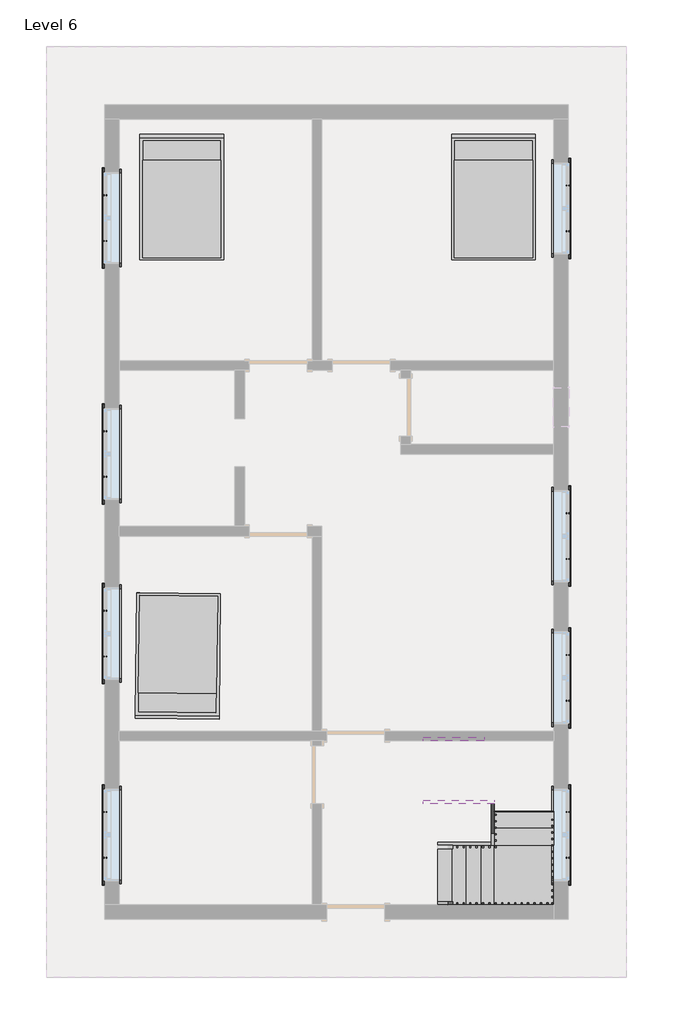
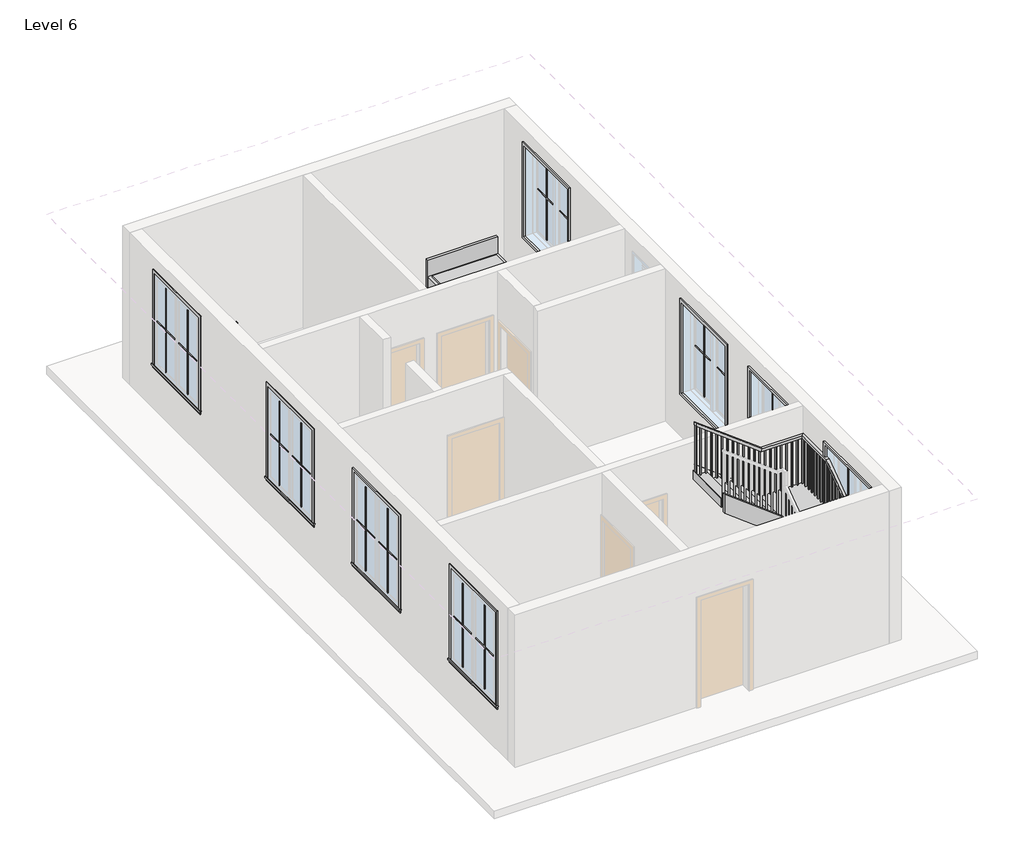
# One storey, part 2 of 2: 32 proxies, 5 members, 3 furniture elements, 1 railing, 1 stair flight.
"""IFC4 building model written with IfcOpenShell, lengths in millimetres."""

from ifc_helpers import new_model, si_unit, frame, origin, place, context, project, spatial, polyline, outline, extrude, faceted_brep, transform, mapped, element, save
from components import muntin_pattern_2x2_muntin_pattern_2x2_bff912c5, muntin_pattern_2x2_muntin_pattern_2x2_c2194282, trim_window_exterior_flat_with_sill_e04b3088, trim_window_interior_flat_picture_frame_2a7685fe, bed_17739_bed_17739_15c61121, stair_flight_c017ec09

model = new_model("IFC4")

# Units and contexts
model_context = context("Model", 3, world=origin())
ifc_project = project(units=[si_unit("LENGTHUNIT", "METRE", prefix="MILLI")], contexts=[model_context])

# Site, building, storey
site = spatial("IfcSite", under=ifc_project)
building = spatial("IfcBuilding", under=site)
storey = spatial("IfcBuildingStorey", under=building, Name="Level 6", Elevation=12801.6)

# Proxies
placement = place(None, origin())
muntin_pattern_2x2_muntin_pattern_2x2_shape = muntin_pattern_2x2_muntin_pattern_2x2_bff912c5(model_context)
element("IfcBuildingElementProxy", 1, Name="Muntin Pattern_2x2 : Muntin Pattern_2x2", ObjectType="Muntin Pattern_2x2 : Muntin Pattern_2x2", at=placement, inside=storey, context=model_context, shape_type="MappedRepresentation", body=[
    mapped(muntin_pattern_2x2_muntin_pattern_2x2_shape, transform((-4903.510885, -5396.5975571, 13785.85), x_axis=(0.0, 1.0, 0.0), y_axis=(-1.0, 0.0, 0.0), z_axis=(0.0, 0.0, 1.0))),
])
element("IfcBuildingElementProxy", 2, Name="Muntin Pattern_2x2 : Muntin Pattern_2x2", ObjectType="Muntin Pattern_2x2 : Muntin Pattern_2x2", at=placement, inside=storey, context=model_context, shape_type="MappedRepresentation", body=[
    mapped(muntin_pattern_2x2_muntin_pattern_2x2_shape, transform((2392.639115, -4675.8725571, 13785.85), x_axis=(0.0, -1.0, 0.0), y_axis=(1.0, 0.0, 0.0), z_axis=(0.0, 0.0, 1.0))),
])
element("IfcBuildingElementProxy", 3, Name="Muntin Pattern_2x2 : Muntin Pattern_2x2", ObjectType="Muntin Pattern_2x2 : Muntin Pattern_2x2", at=placement, inside=storey, context=model_context, shape_type="MappedRepresentation", body=[
    mapped(muntin_pattern_2x2_muntin_pattern_2x2_shape, transform((2392.639115, -2199.3725571, 13785.85), x_axis=(0.0, -1.0, 0.0), y_axis=(1.0, 0.0, 0.0), z_axis=(0.0, 0.0, 1.0))),
])
element("IfcBuildingElementProxy", 4, Name="Muntin Pattern_2x2 : Muntin Pattern_2x2", ObjectType="Muntin Pattern_2x2 : Muntin Pattern_2x2", at=placement, inside=storey, context=model_context, shape_type="MappedRepresentation", body=[
    mapped(muntin_pattern_2x2_muntin_pattern_2x2_shape, transform((2392.639115, 35.8274429, 13785.85), x_axis=(0.0, -1.0, 0.0), y_axis=(1.0, 0.0, 0.0), z_axis=(0.0, 0.0, 1.0))),
])
element("IfcBuildingElementProxy", 5, Name="Muntin Pattern_2x2 : Muntin Pattern_2x2", ObjectType="Muntin Pattern_2x2 : Muntin Pattern_2x2", at=placement, inside=storey, context=model_context, shape_type="MappedRepresentation", body=[
    mapped(muntin_pattern_2x2_muntin_pattern_2x2_shape, transform((-4903.510885, -2221.5975571, 13785.85), x_axis=(0.0, 1.0, 0.0), y_axis=(-1.0, 0.0, 0.0), z_axis=(0.0, 0.0, 1.0))),
])
element("IfcBuildingElementProxy", 6, Name="Muntin Pattern_2x2 : Muntin Pattern_2x2", ObjectType="Muntin Pattern_2x2 : Muntin Pattern_2x2", at=placement, inside=storey, context=model_context, shape_type="MappedRepresentation", body=[
    mapped(muntin_pattern_2x2_muntin_pattern_2x2_shape, transform((-4903.510885, 610.5024429, 13785.85), x_axis=(0.0, 1.0, 0.0), y_axis=(-1.0, 0.0, 0.0), z_axis=(0.0, 0.0, 1.0))),
])
element("IfcBuildingElementProxy", 7, Name="Muntin Pattern_2x2 : Muntin Pattern_2x2", ObjectType="Muntin Pattern_2x2 : Muntin Pattern_2x2", at=placement, inside=storey, context=model_context, shape_type="MappedRepresentation", body=[
    mapped(muntin_pattern_2x2_muntin_pattern_2x2_shape, transform((-4903.510885, 4331.6024429, 13785.85), x_axis=(0.0, 1.0, 0.0), y_axis=(-1.0, 0.0, 0.0), z_axis=(0.0, 0.0, 1.0))),
])
element("IfcBuildingElementProxy", 8, Name="Muntin Pattern_2x2 : Muntin Pattern_2x2", ObjectType="Muntin Pattern_2x2 : Muntin Pattern_2x2", at=placement, inside=storey, context=model_context, shape_type="MappedRepresentation", body=[
    mapped(muntin_pattern_2x2_muntin_pattern_2x2_shape, transform((2392.639115, 5204.7274429, 13785.85), x_axis=(0.0, -1.0, 0.0), y_axis=(1.0, 0.0, 0.0), z_axis=(0.0, 0.0, 1.0))),
])
muntin_pattern_2x2_muntin_pattern_2x2_2_shape = muntin_pattern_2x2_muntin_pattern_2x2_c2194282(model_context)
element("IfcBuildingElementProxy", 9, Name="Muntin Pattern_2x2 : Muntin Pattern_2x2", ObjectType="Muntin Pattern_2x2 : Muntin Pattern_2x2", at=placement, inside=storey, context=model_context, shape_type="MappedRepresentation", body=[
    mapped(muntin_pattern_2x2_muntin_pattern_2x2_2_shape, transform((-4903.510885, -4675.8725571, 13785.85), x_axis=(0.0, -1.0, 0.0), y_axis=(1.0, 0.0, 0.0), z_axis=(0.0, 0.0, 1.0))),
])
element("IfcBuildingElementProxy", 10, Name="Muntin Pattern_2x2 : Muntin Pattern_2x2", ObjectType="Muntin Pattern_2x2 : Muntin Pattern_2x2", at=placement, inside=storey, context=model_context, shape_type="MappedRepresentation", body=[
    mapped(muntin_pattern_2x2_muntin_pattern_2x2_2_shape, transform((2392.639115, -5396.5975571, 13785.85), x_axis=(0.0, 1.0, 0.0), y_axis=(-1.0, 0.0, 0.0), z_axis=(0.0, 0.0, 1.0))),
])
element("IfcBuildingElementProxy", 11, Name="Muntin Pattern_2x2 : Muntin Pattern_2x2", ObjectType="Muntin Pattern_2x2 : Muntin Pattern_2x2", at=placement, inside=storey, context=model_context, shape_type="MappedRepresentation", body=[
    mapped(muntin_pattern_2x2_muntin_pattern_2x2_2_shape, transform((2392.639115, -2920.0975571, 13785.85), x_axis=(0.0, 1.0, 0.0), y_axis=(-1.0, 0.0, 0.0), z_axis=(0.0, 0.0, 1.0))),
])
element("IfcBuildingElementProxy", 12, Name="Muntin Pattern_2x2 : Muntin Pattern_2x2", ObjectType="Muntin Pattern_2x2 : Muntin Pattern_2x2", at=placement, inside=storey, context=model_context, shape_type="MappedRepresentation", body=[
    mapped(muntin_pattern_2x2_muntin_pattern_2x2_2_shape, transform((2392.639115, -684.8975571, 13785.85), x_axis=(0.0, 1.0, 0.0), y_axis=(-1.0, 0.0, 0.0), z_axis=(0.0, 0.0, 1.0))),
])
element("IfcBuildingElementProxy", 13, Name="Muntin Pattern_2x2 : Muntin Pattern_2x2", ObjectType="Muntin Pattern_2x2 : Muntin Pattern_2x2", at=placement, inside=storey, context=model_context, shape_type="MappedRepresentation", body=[
    mapped(muntin_pattern_2x2_muntin_pattern_2x2_2_shape, transform((-4903.510885, -1500.8725571, 13785.85), x_axis=(0.0, -1.0, 0.0), y_axis=(1.0, 0.0, 0.0), z_axis=(0.0, 0.0, 1.0))),
])
element("IfcBuildingElementProxy", 14, Name="Muntin Pattern_2x2 : Muntin Pattern_2x2", ObjectType="Muntin Pattern_2x2 : Muntin Pattern_2x2", at=placement, inside=storey, context=model_context, shape_type="MappedRepresentation", body=[
    mapped(muntin_pattern_2x2_muntin_pattern_2x2_2_shape, transform((-4903.510885, 1331.2274429, 13785.85), x_axis=(0.0, -1.0, 0.0), y_axis=(1.0, 0.0, 0.0), z_axis=(0.0, 0.0, 1.0))),
])
element("IfcBuildingElementProxy", 15, Name="Muntin Pattern_2x2 : Muntin Pattern_2x2", ObjectType="Muntin Pattern_2x2 : Muntin Pattern_2x2", at=placement, inside=storey, context=model_context, shape_type="MappedRepresentation", body=[
    mapped(muntin_pattern_2x2_muntin_pattern_2x2_2_shape, transform((-4903.510885, 5052.3274429, 13785.85), x_axis=(0.0, -1.0, 0.0), y_axis=(1.0, 0.0, 0.0), z_axis=(0.0, 0.0, 1.0))),
])
element("IfcBuildingElementProxy", 16, Name="Muntin Pattern_2x2 : Muntin Pattern_2x2", ObjectType="Muntin Pattern_2x2 : Muntin Pattern_2x2", at=placement, inside=storey, context=model_context, shape_type="MappedRepresentation", body=[
    mapped(muntin_pattern_2x2_muntin_pattern_2x2_2_shape, transform((2392.639115, 4484.0024429, 13785.85), x_axis=(0.0, 1.0, 0.0), y_axis=(-1.0, 0.0, 0.0), z_axis=(0.0, 0.0, 1.0))),
])
trim_window_exterior_flat_with_sill_shape = trim_window_exterior_flat_with_sill_e04b3088(model_context)
element("IfcBuildingElementProxy", 17, Name="Trim-Window-Exterior-Flat : with Sill", ObjectType="Trim-Window-Exterior-Flat : with Sill", at=placement, inside=storey, context=model_context, shape_type="MappedRepresentation", body=[
    mapped(trim_window_exterior_flat_with_sill_shape, transform((-4913.035885, -5036.2350571, 15544.8), x_axis=(0.0, -1.0, 0.0), y_axis=(0.0, 0.0, 1.0), z_axis=(-1.0, 0.0, 0.0))),
])
element("IfcBuildingElementProxy", 18, Name="Trim-Window-Exterior-Flat : with Sill", ObjectType="Trim-Window-Exterior-Flat : with Sill", at=placement, inside=storey, context=model_context, shape_type="MappedRepresentation", body=[
    mapped(trim_window_exterior_flat_with_sill_shape, transform((2402.164115, -5036.2350571, 15544.8), x_axis=(0.0, 1.0, 0.0), y_axis=(0.0, 0.0, 1.0), z_axis=(1.0, 0.0, 0.0))),
])
element("IfcBuildingElementProxy", 19, Name="Trim-Window-Exterior-Flat : with Sill", ObjectType="Trim-Window-Exterior-Flat : with Sill", at=placement, inside=storey, context=model_context, shape_type="MappedRepresentation", body=[
    mapped(trim_window_exterior_flat_with_sill_shape, transform((2402.164115, -2559.7350571, 15544.8), x_axis=(0.0, 1.0, 0.0), y_axis=(0.0, 0.0, 1.0), z_axis=(1.0, 0.0, 0.0))),
])
element("IfcBuildingElementProxy", 20, Name="Trim-Window-Exterior-Flat : with Sill", ObjectType="Trim-Window-Exterior-Flat : with Sill", at=placement, inside=storey, context=model_context, shape_type="MappedRepresentation", body=[
    mapped(trim_window_exterior_flat_with_sill_shape, transform((2402.164115, -324.5350571, 15544.8), x_axis=(0.0, 1.0, 0.0), y_axis=(0.0, 0.0, 1.0), z_axis=(1.0, 0.0, 0.0))),
])
element("IfcBuildingElementProxy", 21, Name="Trim-Window-Exterior-Flat : with Sill", ObjectType="Trim-Window-Exterior-Flat : with Sill", at=placement, inside=storey, context=model_context, shape_type="MappedRepresentation", body=[
    mapped(trim_window_exterior_flat_with_sill_shape, transform((-4913.035885, -1861.2350571, 15544.8), x_axis=(0.0, -1.0, 0.0), y_axis=(0.0, 0.0, 1.0), z_axis=(-1.0, 0.0, 0.0))),
])
element("IfcBuildingElementProxy", 22, Name="Trim-Window-Exterior-Flat : with Sill", ObjectType="Trim-Window-Exterior-Flat : with Sill", at=placement, inside=storey, context=model_context, shape_type="MappedRepresentation", body=[
    mapped(trim_window_exterior_flat_with_sill_shape, transform((-4913.035885, 970.8649429, 15544.8), x_axis=(0.0, -1.0, 0.0), y_axis=(0.0, 0.0, 1.0), z_axis=(-1.0, 0.0, 0.0))),
])
element("IfcBuildingElementProxy", 23, Name="Trim-Window-Exterior-Flat : with Sill", ObjectType="Trim-Window-Exterior-Flat : with Sill", at=placement, inside=storey, context=model_context, shape_type="MappedRepresentation", body=[
    mapped(trim_window_exterior_flat_with_sill_shape, transform((-4913.035885, 4691.9649429, 15544.8), x_axis=(0.0, -1.0, 0.0), y_axis=(0.0, 0.0, 1.0), z_axis=(-1.0, 0.0, 0.0))),
])
element("IfcBuildingElementProxy", 24, Name="Trim-Window-Exterior-Flat : with Sill", ObjectType="Trim-Window-Exterior-Flat : with Sill", at=placement, inside=storey, context=model_context, shape_type="MappedRepresentation", body=[
    mapped(trim_window_exterior_flat_with_sill_shape, transform((2402.164115, 4844.3649429, 15544.8), x_axis=(0.0, 1.0, 0.0), y_axis=(0.0, 0.0, 1.0), z_axis=(1.0, 0.0, 0.0))),
])
trim_window_interior_flat_picture_frame_shape = trim_window_interior_flat_picture_frame_2a7685fe(model_context)
element("IfcBuildingElementProxy", 25, Name="Trim-Window-Interior-Flat : Picture Frame", ObjectType="Trim-Window-Interior-Flat : Picture Frame", at=placement, inside=storey, context=model_context, shape_type="MappedRepresentation", body=[
    mapped(trim_window_interior_flat_picture_frame_shape, transform((-4684.435885, -5036.2350571, 15544.8), x_axis=(0.0, 1.0, 0.0), y_axis=(0.0, 0.0, 1.0), z_axis=(1.0, 0.0, 0.0))),
])
element("IfcBuildingElementProxy", 26, Name="Trim-Window-Interior-Flat : Picture Frame", ObjectType="Trim-Window-Interior-Flat : Picture Frame", at=placement, inside=storey, context=model_context, shape_type="MappedRepresentation", body=[
    mapped(trim_window_interior_flat_picture_frame_shape, transform((2173.564115, -5036.2350571, 15544.8), x_axis=(0.0, -1.0, 0.0), y_axis=(0.0, 0.0, 1.0), z_axis=(-1.0, 0.0, 0.0))),
])
element("IfcBuildingElementProxy", 27, Name="Trim-Window-Interior-Flat : Picture Frame", ObjectType="Trim-Window-Interior-Flat : Picture Frame", at=placement, inside=storey, context=model_context, shape_type="MappedRepresentation", body=[
    mapped(trim_window_interior_flat_picture_frame_shape, transform((2173.564115, -2559.7350571, 15544.8), x_axis=(0.0, -1.0, 0.0), y_axis=(0.0, 0.0, 1.0), z_axis=(-1.0, 0.0, 0.0))),
])
element("IfcBuildingElementProxy", 28, Name="Trim-Window-Interior-Flat : Picture Frame", ObjectType="Trim-Window-Interior-Flat : Picture Frame", at=placement, inside=storey, context=model_context, shape_type="MappedRepresentation", body=[
    mapped(trim_window_interior_flat_picture_frame_shape, transform((2173.564115, -324.5350571, 15544.8), x_axis=(0.0, -1.0, 0.0), y_axis=(0.0, 0.0, 1.0), z_axis=(-1.0, 0.0, 0.0))),
])
element("IfcBuildingElementProxy", 29, Name="Trim-Window-Interior-Flat : Picture Frame", ObjectType="Trim-Window-Interior-Flat : Picture Frame", at=placement, inside=storey, context=model_context, shape_type="MappedRepresentation", body=[
    mapped(trim_window_interior_flat_picture_frame_shape, transform((-4684.435885, -1861.2350571, 15544.8), x_axis=(0.0, 1.0, 0.0), y_axis=(0.0, 0.0, 1.0), z_axis=(1.0, 0.0, 0.0))),
])
element("IfcBuildingElementProxy", 30, Name="Trim-Window-Interior-Flat : Picture Frame", ObjectType="Trim-Window-Interior-Flat : Picture Frame", at=placement, inside=storey, context=model_context, shape_type="MappedRepresentation", body=[
    mapped(trim_window_interior_flat_picture_frame_shape, transform((-4684.435885, 970.8649429, 15544.8), x_axis=(0.0, 1.0, 0.0), y_axis=(0.0, 0.0, 1.0), z_axis=(1.0, 0.0, 0.0))),
])
element("IfcBuildingElementProxy", 31, Name="Trim-Window-Interior-Flat : Picture Frame", ObjectType="Trim-Window-Interior-Flat : Picture Frame", at=placement, inside=storey, context=model_context, shape_type="MappedRepresentation", body=[
    mapped(trim_window_interior_flat_picture_frame_shape, transform((-4684.435885, 4691.9649429, 15544.8), x_axis=(0.0, 1.0, 0.0), y_axis=(0.0, 0.0, 1.0), z_axis=(1.0, 0.0, 0.0))),
])
element("IfcBuildingElementProxy", 32, Name="Trim-Window-Interior-Flat : Picture Frame", ObjectType="Trim-Window-Interior-Flat : Picture Frame", at=placement, inside=storey, context=model_context, shape_type="MappedRepresentation", body=[
    mapped(trim_window_interior_flat_picture_frame_shape, transform((2173.564115, 4844.3649429, 15544.8), x_axis=(0.0, -1.0, 0.0), y_axis=(0.0, 0.0, 1.0), z_axis=(-1.0, 0.0, 0.0))),
])

# Furniture
bed_17739_bed_17739_shape = bed_17739_bed_17739_15c61121(model_context)
element("IfcFurniture", 33, ObjectType="Bed_17739 : Bed_17739", at=placement, inside=storey, context=model_context, shape_type="MappedRepresentation", body=[
    mapped(bed_17739_bed_17739_shape, transform((-3693.835885, 4996.7649429, 12801.6), x_axis=(1.0, 0.0, 0.0), y_axis=(0.0, 1.0, 0.0), z_axis=(0.0, 0.0, 1.0))),
])
element("IfcFurniture", 34, ObjectType="Bed_17739 : Bed_17739", at=placement, inside=storey, context=model_context, shape_type="MappedRepresentation", body=[
    mapped(bed_17739_bed_17739_shape, transform((1221.064115, 4996.7649429, 12801.6), x_axis=(1.0, 0.0, 0.0), y_axis=(0.0, 1.0, 0.0), z_axis=(0.0, 0.0, 1.0))),
])
element("IfcFurniture", 35, ObjectType="Bed_17739 : Bed_17739", at=placement, inside=storey, context=model_context, shape_type="MappedRepresentation", body=[
    mapped(bed_17739_bed_17739_shape, transform((-3756.0321663, -2189.364606, 12801.6), x_axis=(-0.9999334593473937, 0.011535895177843815, 0.0), y_axis=(-0.011535895177843815, -0.9999334593473937, 0.0), z_axis=(0.0, 0.0, 1.0))),
])

# Members
element("IfcMember", 36, ObjectType="Stringer - 2\" Width", at=placement, inside=storey, context=model_context, shape_type="SweptSolid", body=[
    extrude(outline(polyline([(13024.2959685, 344.764115), (12801.6, 344.764115), (12801.6, 555.1685253), (13284.5196844, 1182.964115), (13669.0651993, 1182.964115), (13024.2959685, 344.764115)])), frame((0.0, -5201.3350571, 0.0), z_axis=(0.0, 1.0, 0.0), x_axis=(0.0, 0.0, 1.0)), (0.0, 0.0, 1.0), 50.8),
])
element("IfcMember", 37, ObjectType="Stringer - 2\" Width", at=placement, inside=storey, context=model_context, shape_type="SweptSolid", body=[
    extrude(outline(polyline([(-5201.3350571, 13496.752716), (-5201.3350571, 13871.3225362), (-4540.9350571, 14343.0368219), (-4540.9350571, 13968.4670017), (-5201.3350571, 13496.752716)])), frame((1182.964115, 0.0, 0.0), z_axis=(1.0, 0.0, 0.0), x_axis=(0.0, 1.0, 0.0)), (0.0, 0.0, 1.0), 50.8),
])
element("IfcMember", 38, ObjectType="Stringer - 2\" Width", at=placement, inside=storey, context=model_context, shape_type="SweptSolid", body=[
    extrude(outline(polyline([(14170.7786616, 1233.764115), (14553.9668, 1233.764115), (15405.4715619, 116.164115), (15022.2834236, 116.164115), (14170.7786616, 1233.764115)])), frame((0.0, -4540.9350571, 0.0), z_axis=(0.0, 1.0, 0.0), x_axis=(0.0, 0.0, 1.0)), (0.0, 0.0, 1.0), 50.8),
])
element("IfcMember", 39, ObjectType="Stringer - 2\" Width", at=placement, inside=storey, context=model_context, shape_type="SweptSolid", body=[
    extrude(outline(polyline([(13024.2959685, 344.764115), (12801.6, 344.764115), (12801.6, 555.1685253), (13200.0368219, 1073.1363938), (13200.0368219, 573.2272245), (13024.2959685, 344.764115)])), frame((0.0, -6191.9350571, 0.0), z_axis=(0.0, 1.0, 0.0), x_axis=(0.0, 0.0, 1.0)), (0.0, 0.0, 1.0), 50.8),
])
element("IfcMember", 40, ObjectType="Stringer - 2\" Width", at=placement, inside=storey, context=model_context, shape_type="SweptSolid", body=[
    extrude(outline(polyline([(14676.0384303, 1073.5451003), (15405.4715619, 116.164115), (15022.2834236, 116.164115), (14676.0384303, 570.6106687), (14676.0384303, 1073.5451003)])), frame((0.0, -3550.3350571, 0.0), z_axis=(0.0, 1.0, 0.0), x_axis=(0.0, 0.0, 1.0)), (0.0, 0.0, 1.0), 50.8),
])

# Railing
element("IfcRailing", 41, ObjectType="Handrail - Rectangular", at=placement, inside=storey, context=model_context, shape_type="SolidModel", body=[
    faceted_brep([(344.764115, -6090.3350571, 13885.3333333), (344.764115, -6090.3350571, 13821.4686436), (344.764115, -6141.1350571, 13821.4686436), (344.764115, -6141.1350571, 13885.3333333), (1373.464115, -6090.3350571, 14669.1047619), (1390.6115203, -6090.3350571, 14618.3047619), (1390.6115203, -6141.1350571, 14618.3047619), (1373.464115, -6141.1350571, 14669.1047619), (2122.764115, -6090.3350571, 14669.1047619), (2122.764115, -6090.3350571, 14618.3047619), (2173.564115, -6141.1350571, 14618.3047619), (2173.564115, -6141.1350571, 14669.1047619), (2122.764115, -5289.3883904, 14669.1047619), (2122.764115, -5273.1087657, 14618.3047619), (2173.564115, -5273.1087657, 14618.3047619), (2173.564115, -5289.3883904, 14669.1047619), (2122.764115, -4399.3108146, 15304.8744589), (2122.764115, -4383.0311899, 15254.0744589), (2173.564115, -4383.0311899, 15254.0744589), (2173.564115, -4399.3108146, 15304.8744589), (2122.764115, -3601.1350571, 15304.8744589), (2122.764115, -3601.1350571, 15254.0744589), (2173.564115, -3550.3350571, 15254.0744589), (2173.564115, -3550.3350571, 15304.8744589), (1371.6498293, -3601.1350571, 15304.8744589), (1354.5800477, -3601.1350571, 15254.0744589), (1354.5800477, -3550.3350571, 15254.0744589), (1371.6498293, -3550.3350571, 15304.8744589), (116.164115, -3601.1350571, 16256.0), (116.164115, -3550.3350571, 16256.0), (116.164115, -3550.3350571, 16192.2683472), (116.164115, -3601.1350571, 16192.2683472)], [[[0, 1, 2, 3]], [[1, 0, 4, 5]], [[2, 1, 5, 6]], [[3, 2, 6, 7]], [[0, 3, 7, 4]], [[5, 4, 8, 9]], [[6, 5, 9, 10]], [[7, 6, 10, 11]], [[4, 7, 11, 8]], [[9, 8, 12, 13]], [[10, 9, 13, 14]], [[11, 10, 14, 15]], [[8, 11, 15, 12]], [[13, 12, 16, 17]], [[14, 13, 17, 18]], [[15, 14, 18, 19]], [[12, 15, 19, 16]], [[17, 16, 20, 21]], [[18, 17, 21, 22]], [[19, 18, 22, 23]], [[16, 19, 23, 20]], [[21, 20, 24, 25]], [[22, 21, 25, 26]], [[23, 22, 26, 27]], [[20, 23, 27, 24]], [[28, 29, 30, 31]], [[25, 24, 28, 31]], [[26, 25, 31, 30]], [[27, 26, 30, 29]], [[24, 27, 29, 28]]]),
    extrude(outline(polyline([(16108.0827412, 227.289115), (16122.5145594, 208.239115), (15172.2666667, 208.239115), (15172.2666667, 227.289115), (16108.0827412, 227.289115)])), frame((0.0, -3585.2600571, 0.0), z_axis=(0.0, 1.0, 0.0), x_axis=(0.0, 0.0, 1.0)), (0.0, 0.0, 1.0), 19.05),
    extrude(outline(polyline([(16031.1130442, 328.889115), (16045.5448624, 309.839115), (15172.2666667, 309.839115), (15172.2666667, 328.889115), (16031.1130442, 328.889115)])), frame((0.0, -3585.2600571, 0.0), z_axis=(0.0, 1.0, 0.0), x_axis=(0.0, 0.0, 1.0)), (0.0, 0.0, 1.0), 19.05),
    extrude(outline(polyline([(15954.1433472, 430.489115), (15968.5751654, 411.439115), (15002.9333333, 411.439115), (15002.9333333, 430.489115), (15954.1433472, 430.489115)])), frame((0.0, -3585.2600571, 0.0), z_axis=(0.0, 1.0, 0.0), x_axis=(0.0, 0.0, 1.0)), (0.0, 0.0, 1.0), 19.05),
    extrude(outline(polyline([(15877.1736503, 532.089115), (15891.6054685, 513.039115), (15002.9333333, 513.039115), (15002.9333333, 532.089115), (15877.1736503, 532.089115)])), frame((0.0, -3585.2600571, 0.0), z_axis=(0.0, 1.0, 0.0), x_axis=(0.0, 0.0, 1.0)), (0.0, 0.0, 1.0), 19.05),
    extrude(outline(polyline([(15800.2039533, 633.689115), (15814.6357715, 614.639115), (14833.6, 614.639115), (14833.6, 633.689115), (15800.2039533, 633.689115)])), frame((0.0, -3585.2600571, 0.0), z_axis=(0.0, 1.0, 0.0), x_axis=(0.0, 0.0, 1.0)), (0.0, 0.0, 1.0), 19.05),
    extrude(outline(polyline([(15723.2342563, 735.289115), (15737.6660745, 716.239115), (14833.6, 716.239115), (14833.6, 735.289115), (15723.2342563, 735.289115)])), frame((0.0, -3585.2600571, 0.0), z_axis=(0.0, 1.0, 0.0), x_axis=(0.0, 0.0, 1.0)), (0.0, 0.0, 1.0), 19.05),
    extrude(outline(polyline([(15646.2645594, 836.889115), (15660.6963775, 817.839115), (14664.2666667, 817.839115), (14664.2666667, 836.889115), (15646.2645594, 836.889115)])), frame((0.0, -3585.2600571, 0.0), z_axis=(0.0, 1.0, 0.0), x_axis=(0.0, 0.0, 1.0)), (0.0, 0.0, 1.0), 19.05),
    extrude(outline(polyline([(15569.2948624, 938.489115), (15583.7266806, 919.439115), (14664.2666667, 919.439115), (14664.2666667, 938.489115), (15569.2948624, 938.489115)])), frame((0.0, -3585.2600571, 0.0), z_axis=(0.0, 1.0, 0.0), x_axis=(0.0, 0.0, 1.0)), (0.0, 0.0, 1.0), 19.05),
    extrude(outline(polyline([(15492.3251654, 1040.089115), (15506.7569836, 1021.039115), (14664.2666667, 1021.039115), (14664.2666667, 1040.089115), (15492.3251654, 1040.089115)])), frame((0.0, -3585.2600571, 0.0), z_axis=(0.0, 1.0, 0.0), x_axis=(0.0, 0.0, 1.0)), (0.0, 0.0, 1.0), 19.05),
    extrude(outline(polyline([(15415.3554685, 1141.689115), (15429.7872866, 1122.639115), (14494.9333333, 1122.639115), (14494.9333333, 1141.689115), (15415.3554685, 1141.689115)])), frame((0.0, -3585.2600571, 0.0), z_axis=(0.0, 1.0, 0.0), x_axis=(0.0, 0.0, 1.0)), (0.0, 0.0, 1.0), 19.05),
    extrude(outline(polyline([(15338.3857715, 1243.289115), (15352.8175897, 1224.239115), (14494.9333333, 1224.239115), (14494.9333333, 1243.289115), (15338.3857715, 1243.289115)])), frame((0.0, -3585.2600571, 0.0), z_axis=(0.0, 1.0, 0.0), x_axis=(0.0, 0.0, 1.0)), (0.0, 0.0, 1.0), 19.05),
    extrude(outline(polyline([(15261.4160745, 1344.889115), (15275.8478927, 1325.839115), (14325.6, 1325.839115), (14325.6, 1344.889115), (15261.4160745, 1344.889115)])), frame((0.0, -3585.2600571, 0.0), z_axis=(0.0, 1.0, 0.0), x_axis=(0.0, 0.0, 1.0)), (0.0, 0.0, 1.0), 19.05),
    extrude(outline(polyline([(1446.489115, -3566.2100571), (1446.489115, -3585.2600571), (1427.439115, -3585.2600571), (1427.439115, -3566.2100571), (1446.489115, -3566.2100571)])), frame((0.0, 0.0, 14325.6), z_axis=(0.0, 0.0, 1.0), x_axis=(1.0, 0.0, 0.0)), (0.0, 0.0, 1.0), 928.4744589),
    extrude(outline(polyline([(1548.089115, -3566.2100571), (1548.089115, -3585.2600571), (1529.039115, -3585.2600571), (1529.039115, -3566.2100571), (1548.089115, -3566.2100571)])), frame((0.0, 0.0, 14325.6), z_axis=(0.0, 0.0, 1.0), x_axis=(1.0, 0.0, 0.0)), (0.0, 0.0, 1.0), 928.4744589),
    extrude(outline(polyline([(1649.689115, -3566.2100571), (1649.689115, -3585.2600571), (1630.639115, -3585.2600571), (1630.639115, -3566.2100571), (1649.689115, -3566.2100571)])), frame((0.0, 0.0, 14325.6), z_axis=(0.0, 0.0, 1.0), x_axis=(1.0, 0.0, 0.0)), (0.0, 0.0, 1.0), 928.4744589),
    extrude(outline(polyline([(1751.289115, -3566.2100571), (1751.289115, -3585.2600571), (1732.239115, -3585.2600571), (1732.239115, -3566.2100571), (1751.289115, -3566.2100571)])), frame((0.0, 0.0, 14325.6), z_axis=(0.0, 0.0, 1.0), x_axis=(1.0, 0.0, 0.0)), (0.0, 0.0, 1.0), 928.4744589),
    extrude(outline(polyline([(1852.889115, -3566.2100571), (1852.889115, -3585.2600571), (1833.839115, -3585.2600571), (1833.839115, -3566.2100571), (1852.889115, -3566.2100571)])), frame((0.0, 0.0, 14325.6), z_axis=(0.0, 0.0, 1.0), x_axis=(1.0, 0.0, 0.0)), (0.0, 0.0, 1.0), 928.4744589),
    extrude(outline(polyline([(1954.489115, -3566.2100571), (1954.489115, -3585.2600571), (1935.439115, -3585.2600571), (1935.439115, -3566.2100571), (1954.489115, -3566.2100571)])), frame((0.0, 0.0, 14325.6), z_axis=(0.0, 0.0, 1.0), x_axis=(1.0, 0.0, 0.0)), (0.0, 0.0, 1.0), 928.4744589),
    extrude(outline(polyline([(2056.089115, -3566.2100571), (2056.089115, -3585.2600571), (2037.039115, -3585.2600571), (2037.039115, -3566.2100571), (2056.089115, -3566.2100571)])), frame((0.0, 0.0, 14325.6), z_axis=(0.0, 0.0, 1.0), x_axis=(1.0, 0.0, 0.0)), (0.0, 0.0, 1.0), 928.4744589),
    extrude(outline(polyline([(2157.689115, -3686.8600571), (2138.639115, -3686.8600571), (2138.639115, -3667.8100571), (2157.689115, -3667.8100571), (2157.689115, -3686.8600571)])), frame((0.0, 0.0, 14325.6), z_axis=(0.0, 0.0, 1.0), x_axis=(1.0, 0.0, 0.0)), (0.0, 0.0, 1.0), 928.4744589),
    extrude(outline(polyline([(2157.689115, -3788.4600571), (2138.639115, -3788.4600571), (2138.639115, -3769.4100571), (2157.689115, -3769.4100571), (2157.689115, -3788.4600571)])), frame((0.0, 0.0, 14325.6), z_axis=(0.0, 0.0, 1.0), x_axis=(1.0, 0.0, 0.0)), (0.0, 0.0, 1.0), 928.4744589),
    extrude(outline(polyline([(2157.689115, -3890.0600571), (2138.639115, -3890.0600571), (2138.639115, -3871.0100571), (2157.689115, -3871.0100571), (2157.689115, -3890.0600571)])), frame((0.0, 0.0, 14325.6), z_axis=(0.0, 0.0, 1.0), x_axis=(1.0, 0.0, 0.0)), (0.0, 0.0, 1.0), 928.4744589),
    extrude(outline(polyline([(2157.689115, -3991.6600571), (2138.639115, -3991.6600571), (2138.639115, -3972.6100571), (2157.689115, -3972.6100571), (2157.689115, -3991.6600571)])), frame((0.0, 0.0, 14325.6), z_axis=(0.0, 0.0, 1.0), x_axis=(1.0, 0.0, 0.0)), (0.0, 0.0, 1.0), 928.4744589),
    extrude(outline(polyline([(2157.689115, -4093.2600571), (2138.639115, -4093.2600571), (2138.639115, -4074.2100571), (2157.689115, -4074.2100571), (2157.689115, -4093.2600571)])), frame((0.0, 0.0, 14325.6), z_axis=(0.0, 0.0, 1.0), x_axis=(1.0, 0.0, 0.0)), (0.0, 0.0, 1.0), 928.4744589),
    extrude(outline(polyline([(2157.689115, -4194.8600571), (2138.639115, -4194.8600571), (2138.639115, -4175.8100571), (2157.689115, -4175.8100571), (2157.689115, -4194.8600571)])), frame((0.0, 0.0, 14325.6), z_axis=(0.0, 0.0, 1.0), x_axis=(1.0, 0.0, 0.0)), (0.0, 0.0, 1.0), 928.4744589),
    extrude(outline(polyline([(2157.689115, -4296.4600571), (2138.639115, -4296.4600571), (2138.639115, -4277.4100571), (2157.689115, -4277.4100571), (2157.689115, -4296.4600571)])), frame((0.0, 0.0, 14325.6), z_axis=(0.0, 0.0, 1.0), x_axis=(1.0, 0.0, 0.0)), (0.0, 0.0, 1.0), 928.4744589),
    extrude(outline(polyline([(2157.689115, -4398.0600571), (2138.639115, -4398.0600571), (2138.639115, -4379.0100571), (2157.689115, -4379.0100571), (2157.689115, -4398.0600571)])), frame((0.0, 0.0, 14325.6), z_axis=(0.0, 0.0, 1.0), x_axis=(1.0, 0.0, 0.0)), (0.0, 0.0, 1.0), 928.4744589),
    extrude(outline(polyline([(-4499.6600571, 15170.7681252), (-4480.6100571, 15184.3752681), (-4480.6100571, 14325.6), (-4499.6600571, 14325.6), (-4499.6600571, 15170.7681252)])), frame((2138.639115, 0.0, 0.0), z_axis=(1.0, 0.0, 0.0), x_axis=(0.0, 1.0, 0.0)), (0.0, 0.0, 1.0), 19.05),
    extrude(outline(polyline([(-4601.2600571, 15098.1966966), (-4582.2100571, 15111.8038395), (-4582.2100571, 14156.2666667), (-4601.2600571, 14156.2666667), (-4601.2600571, 15098.1966966)])), frame((2138.639115, 0.0, 0.0), z_axis=(1.0, 0.0, 0.0), x_axis=(0.0, 1.0, 0.0)), (0.0, 0.0, 1.0), 19.05),
    extrude(outline(polyline([(-4702.8600571, 15025.6252681), (-4683.8100571, 15039.2324109), (-4683.8100571, 14156.2666667), (-4702.8600571, 14156.2666667), (-4702.8600571, 15025.6252681)])), frame((2138.639115, 0.0, 0.0), z_axis=(1.0, 0.0, 0.0), x_axis=(0.0, 1.0, 0.0)), (0.0, 0.0, 1.0), 19.05),
    extrude(outline(polyline([(-4804.4600571, 14953.0538395), (-4785.4100571, 14966.6609823), (-4785.4100571, 13986.9333333), (-4804.4600571, 13986.9333333), (-4804.4600571, 14953.0538395)])), frame((2138.639115, 0.0, 0.0), z_axis=(1.0, 0.0, 0.0), x_axis=(0.0, 1.0, 0.0)), (0.0, 0.0, 1.0), 19.05),
    extrude(outline(polyline([(-4906.0600571, 14880.4824109), (-4887.0100571, 14894.0895538), (-4887.0100571, 13986.9333333), (-4906.0600571, 13986.9333333), (-4906.0600571, 14880.4824109)])), frame((2138.639115, 0.0, 0.0), z_axis=(1.0, 0.0, 0.0), x_axis=(0.0, 1.0, 0.0)), (0.0, 0.0, 1.0), 19.05),
    extrude(outline(polyline([(-5007.6600571, 14807.9109823), (-4988.6100571, 14821.5181252), (-4988.6100571, 13817.6), (-5007.6600571, 13817.6), (-5007.6600571, 14807.9109823)])), frame((2138.639115, 0.0, 0.0), z_axis=(1.0, 0.0, 0.0), x_axis=(0.0, 1.0, 0.0)), (0.0, 0.0, 1.0), 19.05),
    extrude(outline(polyline([(-5109.2600571, 14735.3395538), (-5090.2100571, 14748.9466966), (-5090.2100571, 13817.6), (-5109.2600571, 13817.6), (-5109.2600571, 14735.3395538)])), frame((2138.639115, 0.0, 0.0), z_axis=(1.0, 0.0, 0.0), x_axis=(0.0, 1.0, 0.0)), (0.0, 0.0, 1.0), 19.05),
    extrude(outline(polyline([(-5210.8600571, 14662.7681252), (-5191.8100571, 14676.3752681), (-5191.8100571, 13817.6), (-5210.8600571, 13817.6), (-5210.8600571, 14662.7681252)])), frame((2138.639115, 0.0, 0.0), z_axis=(1.0, 0.0, 0.0), x_axis=(0.0, 1.0, 0.0)), (0.0, 0.0, 1.0), 19.05),
    extrude(outline(polyline([(2157.689115, -5312.4600571), (2138.639115, -5312.4600571), (2138.639115, -5293.4100571), (2157.689115, -5293.4100571), (2157.689115, -5312.4600571)])), frame((0.0, 0.0, 13648.2666667), z_axis=(0.0, 0.0, 1.0), x_axis=(1.0, 0.0, 0.0)), (0.0, 0.0, 1.0), 970.0380952),
    extrude(outline(polyline([(2157.689115, -5414.0600571), (2138.639115, -5414.0600571), (2138.639115, -5395.0100571), (2157.689115, -5395.0100571), (2157.689115, -5414.0600571)])), frame((0.0, 0.0, 13648.2666667), z_axis=(0.0, 0.0, 1.0), x_axis=(1.0, 0.0, 0.0)), (0.0, 0.0, 1.0), 970.0380952),
    extrude(outline(polyline([(2157.689115, -5515.6600571), (2138.639115, -5515.6600571), (2138.639115, -5496.6100571), (2157.689115, -5496.6100571), (2157.689115, -5515.6600571)])), frame((0.0, 0.0, 13648.2666667), z_axis=(0.0, 0.0, 1.0), x_axis=(1.0, 0.0, 0.0)), (0.0, 0.0, 1.0), 970.0380952),
    extrude(outline(polyline([(2157.689115, -5617.2600571), (2138.639115, -5617.2600571), (2138.639115, -5598.2100571), (2157.689115, -5598.2100571), (2157.689115, -5617.2600571)])), frame((0.0, 0.0, 13648.2666667), z_axis=(0.0, 0.0, 1.0), x_axis=(1.0, 0.0, 0.0)), (0.0, 0.0, 1.0), 970.0380952),
    extrude(outline(polyline([(2157.689115, -5718.8600571), (2138.639115, -5718.8600571), (2138.639115, -5699.8100571), (2157.689115, -5699.8100571), (2157.689115, -5718.8600571)])), frame((0.0, 0.0, 13648.2666667), z_axis=(0.0, 0.0, 1.0), x_axis=(1.0, 0.0, 0.0)), (0.0, 0.0, 1.0), 970.0380952),
    extrude(outline(polyline([(2157.689115, -5820.4600571), (2138.639115, -5820.4600571), (2138.639115, -5801.4100571), (2157.689115, -5801.4100571), (2157.689115, -5820.4600571)])), frame((0.0, 0.0, 13648.2666667), z_axis=(0.0, 0.0, 1.0), x_axis=(1.0, 0.0, 0.0)), (0.0, 0.0, 1.0), 970.0380952),
    extrude(outline(polyline([(2157.689115, -5922.0600571), (2138.639115, -5922.0600571), (2138.639115, -5903.0100571), (2157.689115, -5903.0100571), (2157.689115, -5922.0600571)])), frame((0.0, 0.0, 13648.2666667), z_axis=(0.0, 0.0, 1.0), x_axis=(1.0, 0.0, 0.0)), (0.0, 0.0, 1.0), 970.0380952),
    extrude(outline(polyline([(2157.689115, -6023.6600571), (2138.639115, -6023.6600571), (2138.639115, -6004.6100571), (2157.689115, -6004.6100571), (2157.689115, -6023.6600571)])), frame((0.0, 0.0, 13648.2666667), z_axis=(0.0, 0.0, 1.0), x_axis=(1.0, 0.0, 0.0)), (0.0, 0.0, 1.0), 970.0380952),
    extrude(outline(polyline([(2062.439115, -6125.2600571), (2062.439115, -6106.2100571), (2081.489115, -6106.2100571), (2081.489115, -6125.2600571), (2062.439115, -6125.2600571)])), frame((0.0, 0.0, 13648.2666667), z_axis=(0.0, 0.0, 1.0), x_axis=(1.0, 0.0, 0.0)), (0.0, 0.0, 1.0), 970.0380952),
    extrude(outline(polyline([(1960.839115, -6125.2600571), (1960.839115, -6106.2100571), (1979.889115, -6106.2100571), (1979.889115, -6125.2600571), (1960.839115, -6125.2600571)])), frame((0.0, 0.0, 13648.2666667), z_axis=(0.0, 0.0, 1.0), x_axis=(1.0, 0.0, 0.0)), (0.0, 0.0, 1.0), 970.0380952),
    extrude(outline(polyline([(1859.239115, -6125.2600571), (1859.239115, -6106.2100571), (1878.289115, -6106.2100571), (1878.289115, -6125.2600571), (1859.239115, -6125.2600571)])), frame((0.0, 0.0, 13648.2666667), z_axis=(0.0, 0.0, 1.0), x_axis=(1.0, 0.0, 0.0)), (0.0, 0.0, 1.0), 970.0380952),
    extrude(outline(polyline([(1757.639115, -6125.2600571), (1757.639115, -6106.2100571), (1776.689115, -6106.2100571), (1776.689115, -6125.2600571), (1757.639115, -6125.2600571)])), frame((0.0, 0.0, 13648.2666667), z_axis=(0.0, 0.0, 1.0), x_axis=(1.0, 0.0, 0.0)), (0.0, 0.0, 1.0), 970.0380952),
    extrude(outline(polyline([(1656.039115, -6125.2600571), (1656.039115, -6106.2100571), (1675.089115, -6106.2100571), (1675.089115, -6125.2600571), (1656.039115, -6125.2600571)])), frame((0.0, 0.0, 13648.2666667), z_axis=(0.0, 0.0, 1.0), x_axis=(1.0, 0.0, 0.0)), (0.0, 0.0, 1.0), 970.0380952),
    extrude(outline(polyline([(1554.439115, -6125.2600571), (1554.439115, -6106.2100571), (1573.489115, -6106.2100571), (1573.489115, -6125.2600571), (1554.439115, -6125.2600571)])), frame((0.0, 0.0, 13648.2666667), z_axis=(0.0, 0.0, 1.0), x_axis=(1.0, 0.0, 0.0)), (0.0, 0.0, 1.0), 970.0380952),
    extrude(outline(polyline([(1452.839115, -6125.2600571), (1452.839115, -6106.2100571), (1471.889115, -6106.2100571), (1471.889115, -6125.2600571), (1452.839115, -6125.2600571)])), frame((0.0, 0.0, 13648.2666667), z_axis=(0.0, 0.0, 1.0), x_axis=(1.0, 0.0, 0.0)), (0.0, 0.0, 1.0), 970.0380952),
    extrude(outline(polyline([(14602.8210246, 1370.289115), (14588.3067388, 1351.239115), (13648.2666667, 1351.239115), (13648.2666667, 1370.289115), (14602.8210246, 1370.289115)])), frame((0.0, -6125.2600571, 0.0), z_axis=(0.0, 1.0, 0.0), x_axis=(0.0, 0.0, 1.0)), (0.0, 0.0, 1.0), 19.05),
    extrude(outline(polyline([(14525.4115007, 1268.689115), (14510.897215, 1249.639115), (13648.2666667, 1249.639115), (13648.2666667, 1268.689115), (14525.4115007, 1268.689115)])), frame((0.0, -6125.2600571, 0.0), z_axis=(0.0, 1.0, 0.0), x_axis=(0.0, 0.0, 1.0)), (0.0, 0.0, 1.0), 19.05),
    extrude(outline(polyline([(14448.0019769, 1167.089115), (14433.4876912, 1148.039115), (13478.9333333, 1148.039115), (13478.9333333, 1167.089115), (14448.0019769, 1167.089115)])), frame((0.0, -6125.2600571, 0.0), z_axis=(0.0, 1.0, 0.0), x_axis=(0.0, 0.0, 1.0)), (0.0, 0.0, 1.0), 19.05),
    extrude(outline(polyline([(14370.5924531, 1065.489115), (14356.0781674, 1046.439115), (13478.9333333, 1046.439115), (13478.9333333, 1065.489115), (14370.5924531, 1065.489115)])), frame((0.0, -6125.2600571, 0.0), z_axis=(0.0, 1.0, 0.0), x_axis=(0.0, 0.0, 1.0)), (0.0, 0.0, 1.0), 19.05),
    extrude(outline(polyline([(14293.1829293, 963.889115), (14278.6686436, 944.839115), (13309.6, 944.839115), (13309.6, 963.889115), (14293.1829293, 963.889115)])), frame((0.0, -6125.2600571, 0.0), z_axis=(0.0, 1.0, 0.0), x_axis=(0.0, 0.0, 1.0)), (0.0, 0.0, 1.0), 19.05),
    extrude(outline(polyline([(14215.7734055, 862.289115), (14201.2591198, 843.239115), (13309.6, 843.239115), (13309.6, 862.289115), (14215.7734055, 862.289115)])), frame((0.0, -6125.2600571, 0.0), z_axis=(0.0, 1.0, 0.0), x_axis=(0.0, 0.0, 1.0)), (0.0, 0.0, 1.0), 19.05),
    extrude(outline(polyline([(14138.3638817, 760.689115), (14123.849596, 741.639115), (13140.2666667, 741.639115), (13140.2666667, 760.689115), (14138.3638817, 760.689115)])), frame((0.0, -6125.2600571, 0.0), z_axis=(0.0, 1.0, 0.0), x_axis=(0.0, 0.0, 1.0)), (0.0, 0.0, 1.0), 19.05),
    extrude(outline(polyline([(14060.9543579, 659.089115), (14046.4400722, 640.039115), (13140.2666667, 640.039115), (13140.2666667, 659.089115), (14060.9543579, 659.089115)])), frame((0.0, -6125.2600571, 0.0), z_axis=(0.0, 1.0, 0.0), x_axis=(0.0, 0.0, 1.0)), (0.0, 0.0, 1.0), 19.05),
    extrude(outline(polyline([(13983.5448341, 557.489115), (13969.0305484, 538.439115), (12970.9333333, 538.439115), (12970.9333333, 557.489115), (13983.5448341, 557.489115)])), frame((0.0, -6125.2600571, 0.0), z_axis=(0.0, 1.0, 0.0), x_axis=(0.0, 0.0, 1.0)), (0.0, 0.0, 1.0), 19.05),
    extrude(outline(polyline([(13906.1353103, 455.889115), (13891.6210246, 436.839115), (12970.9333333, 436.839115), (12970.9333333, 455.889115), (13906.1353103, 455.889115)])), frame((0.0, -6125.2600571, 0.0), z_axis=(0.0, 1.0, 0.0), x_axis=(0.0, 0.0, 1.0)), (0.0, 0.0, 1.0), 19.05),
    extrude(outline(polyline([(2157.689115, -3585.2600571), (2138.639115, -3585.2600571), (2138.639115, -3566.2100571), (2157.689115, -3566.2100571), (2157.689115, -3585.2600571)])), frame((0.0, 0.0, 14325.6), z_axis=(0.0, 0.0, 1.0), x_axis=(1.0, 0.0, 0.0)), (0.0, 0.0, 1.0), 928.4744589),
    extrude(outline(polyline([(2138.639115, -6125.2600571), (2138.639115, -6106.2100571), (2157.689115, -6106.2100571), (2157.689115, -6125.2600571), (2138.639115, -6125.2600571)])), frame((0.0, 0.0, 13648.2666667), z_axis=(0.0, 0.0, 1.0), x_axis=(1.0, 0.0, 0.0)), (0.0, 0.0, 1.0), 970.0380952),
    extrude(outline(polyline([(16177.8365291, 135.214115), (16192.2683472, 116.164115), (15172.2666667, 116.164115), (15172.2666667, 135.214115), (16177.8365291, 135.214115)])), frame((0.0, -3585.2600571, 0.0), z_axis=(0.0, 1.0, 0.0), x_axis=(0.0, 0.0, 1.0)), (0.0, 0.0, 1.0), 19.05),
    extrude(outline(polyline([(13835.9829293, 363.814115), (13821.4686436, 344.764115), (12970.9333333, 344.764115), (12970.9333333, 363.814115), (13835.9829293, 363.814115)])), frame((0.0, -6125.2600571, 0.0), z_axis=(0.0, 1.0, 0.0), x_axis=(0.0, 0.0, 1.0)), (0.0, 0.0, 1.0), 19.05),
])

# Stair flight
stair_flight_shape = stair_flight_c017ec09(model_context)
element("IfcStairFlight", 42, ObjectType="2\" Tread 1\" Nosing 1/4\" Riser", at=placement, inside=storey, context=model_context, shape_type="MappedRepresentation", body=[
    mapped(stair_flight_shape, transform((0.0, 0.0, 0.0), x_axis=(1.0, 0.0, 0.0), y_axis=(0.0, 1.0, 0.0), z_axis=(0.0, 0.0, 1.0))),
])

save(model, "model.ifc")

# Revit data of these elements
# Type "Muntin Pattern_2x2 : Muntin Pattern_2x2"
#   Width [instance default] = 4' - 0"
#   Thickness = 0' - 0 1/2"
#   Height [instance default] = 4' - 0"
#   Distance = 0' - 0 3/4"
#   Interior Material [instance default] = none
#   Exterior Material [instance default] = none
#   Default Elevation = 0
# Type "Trim-Window-Exterior-Flat : with Sill"
#   Trim Width = 0' - 2 1/4"
#   Trim Thickness_Picture Frame = 0' - 1 1/4"
#   Trim Thickness_with Sill = 0' - 0 3/4"
#   Sill Thickness = 0' - 1 1/4"
#   Opening Width [instance default] = 2' - 0"
#   Opening Height [instance default] = 3' - 0"
#   Default Elevation = 4' - 0"
#   Sill = yes
#   Picture Frame = no
#   Trim Material [instance default] = none
# Type "Trim-Window-Interior-Flat : Picture Frame"
#   Trim Thickness_Picture Frame = 0' - 1 1/4"
#   Trim Width = 0' - 2 1/4"
#   Trim Thickness_with Sill = 0' - 0 3/4"
#   Sill Thickness = 0' - 1 1/4"
#   Opening Width [instance default] = 2' - 0"
#   Opening Height [instance default] = 3' - 0"
#   Default Elevation = 4' - 0"
#   Sill = no
#   Picture Frame = yes
#   Trim Material [instance default] = none
# Type "Bed_17739 : Bed_17739"
#   Default Elevation = 0
# Type "Handrail - Rectangular"
#   Assembly Code = "C2010400"
#   built-in parameter 1008612 = 0.0416667 (stored number, unit not read)
#   built-in parameter 1008611 = 0.0416667 (stored number, unit not read)
#   built-in parameter 1008609 = 0.333333 (stored number, unit not read)
#   built-in parameter 1008604 = 0.166667 (stored number, unit not read)
#   built-in parameter 1008603 = 0.166667 (stored number, unit not read)
#   Railing Height = 3' - 0"
#   built-in parameter 1008630 = 2
#   built-in parameter 1008610 = 2
#   built-in parameter 1008618 = Baluster - Square : 3/4"
# Elements 1, 2, 3, 4, 5, 6, 7, 8, 9, 10, 11, 12, 13, 14, 15, 16 (IfcBuildingElementProxy, "Muntin Pattern_2x2 : Muntin Pattern_2x2")
#   Width = 1' - 11 1/8"
#   Height = 5' - 6 1/2"
#   Interior Material = Wood - Stained
#   Exterior Material = Clad - White
#   Phase Created = New Construction
#   Materials on its faces: "Clad - White", "Wood - Stained"
# Elements 17, 18, 19, 20, 21, 22, 23, 24 (IfcBuildingElementProxy, "Trim-Window-Exterior-Flat : with Sill")
#   Opening Width = 4' - 9"
#   Opening Height = 6' - 0"
#   Trim Material = Clad - White
#   Phase Created = New Construction
#   Materials on its faces: "Clad - White"
# Elements 25, 26, 27, 28, 29, 30, 31, 32 (IfcBuildingElementProxy, "Trim-Window-Interior-Flat : Picture Frame")
#   Opening Width = 4' - 9"
#   Opening Height = 6' - 0"
#   Trim Material = Wood - Stained
#   Phase Created = New Construction
#   Materials on its faces: "Wood - Stained"
# Elements 33, 34, 35 (IfcFurniture, "Bed_17739 : Bed_17739")
#   Phase Created = New Construction
#   Materials on its faces: "legs", "sheets", "bed frame", "Blanket"
# Elements 36, 37, 38, 39, 40 (IfcMember, "Stringer - 2\" Width")
#   Phase Created = New Construction
# Element 41 (IfcRailing, "Handrail - Rectangular")
#   Phase Created = New Construction
# Element 42 (IfcStairFlight, "2\" Tread 1\" Nosing 1/4\" Riser")
#   Phase Created = New Construction
# Materials
#   "Clad - White": class "Wood", colour RGB 242 242 238, transparency 0, Cost = 0
#   "Wood - Stained": class "Wood", colour RGB 224 178 126, transparency 0, Cost = 0
#   "legs": colour RGB 90 73 37, transparency 0, Cost = 0
#   "sheets": colour RGB 200 195 176, transparency 0, Cost = 0
#   "bed frame": colour RGB 90 73 37, transparency 0, Cost = 0
#   "Blanket": class "System", colour RGB 59 0 1, transparency 0, Cost = 0
